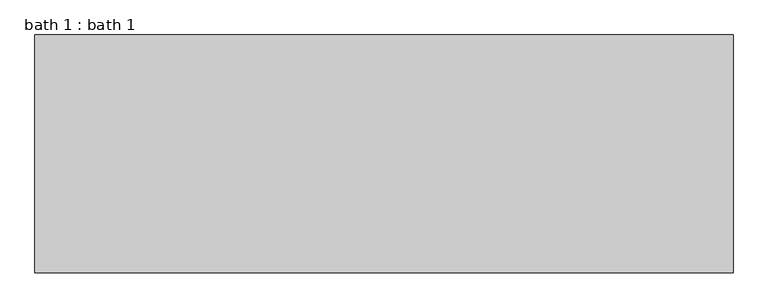
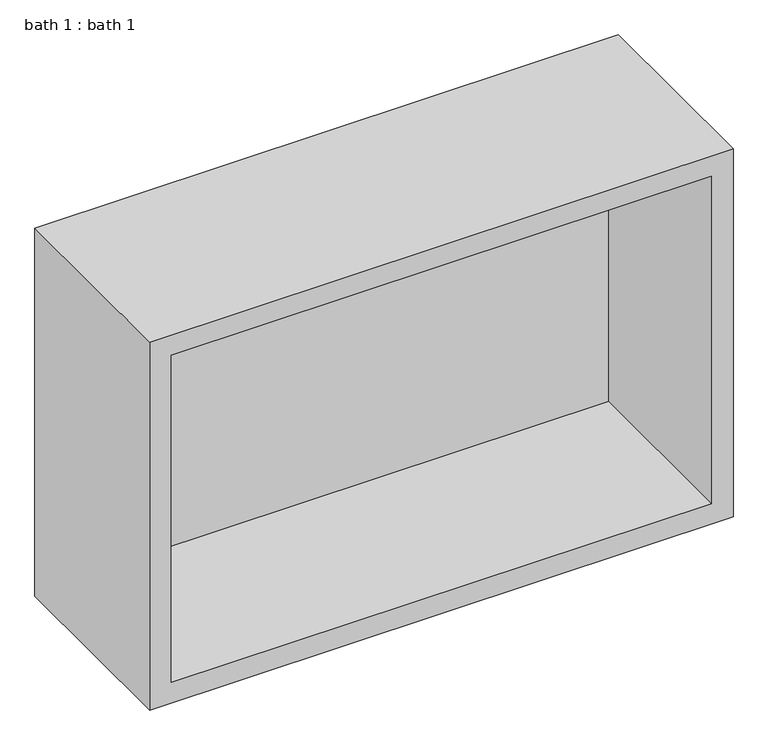
"""IFC4 building model written with IfcOpenShell, lengths in millimetres: proxy geometry, bath 1 : bath 1."""

from ifc_helpers import new_model, si_unit, origin, place, context, project, spatial, faceted_brep, source, transform, mapped, element, save


def bath_1_bath_1_5f45cd17(model_context):
    return source(origin(), model_context, "Body", "Brep", [
        faceted_brep([(-1385.5005972, -3141.3129108, 0.0), (-1385.5005972, -3608.3639228, 0.0), (-2757.1005972, -3608.3639228, 0.0), (-2757.1005972, -3141.3129108, 0.0), (-1385.5005972, -3141.3129108, 914.4), (-2757.1005972, -3141.3129108, 914.4), (-2757.1005972, -3608.3639228, 914.4), (-1385.5005972, -3608.3639228, 914.4), (-2706.3005972, -3608.3639228, 863.6), (-1436.3005972, -3608.3639228, 863.6), (-1436.3005972, -3608.3639228, 50.8), (-2706.3005972, -3608.3639228, 50.8), (-2706.3005972, -3189.6077009, 863.6), (-2706.3005972, -3189.6077009, 50.8), (-1436.3005972, -3189.6077009, 50.8), (-1436.3005972, -3189.6077009, 863.6)], [[[0, 1, 2, 3]], [[4, 5, 6, 7]], [[0, 3, 5, 4]], [[3, 2, 6, 5]], [[2, 1, 7, 6], [8, 9, 10, 11]], [[1, 0, 4, 7]], [[12, 13, 14, 15]], [[12, 15, 9, 8]], [[15, 14, 10, 9]], [[14, 13, 11, 10]], [[13, 12, 8, 11]]]),
    ])


if __name__ == "__main__":
    model = new_model("IFC4")
    model_context = context("Model", 3, world=origin())
    ifc_project = project(units=[si_unit("LENGTHUNIT", "METRE", prefix="MILLI")], contexts=[model_context])
    site = spatial("IfcSite", under=ifc_project)
    building = spatial("IfcBuilding", under=site)
    placement = place(None, origin())
    bath_1_bath_1_shape = bath_1_bath_1_5f45cd17(model_context)
    element("IfcBuildingElementProxy", 1, Name="bath 1 : bath 1", ObjectType="bath 1 : bath 1", at=placement, inside=building, context=model_context, shape_type="MappedRepresentation", body=[
        mapped(bath_1_bath_1_shape, transform((0.0, 0.0, 0.0), x_axis=(1.0, 0.0, 0.0), y_axis=(0.0, 1.0, 0.0), z_axis=(0.0, 0.0, 1.0))),
    ])
    save(model, "model.ifc")
